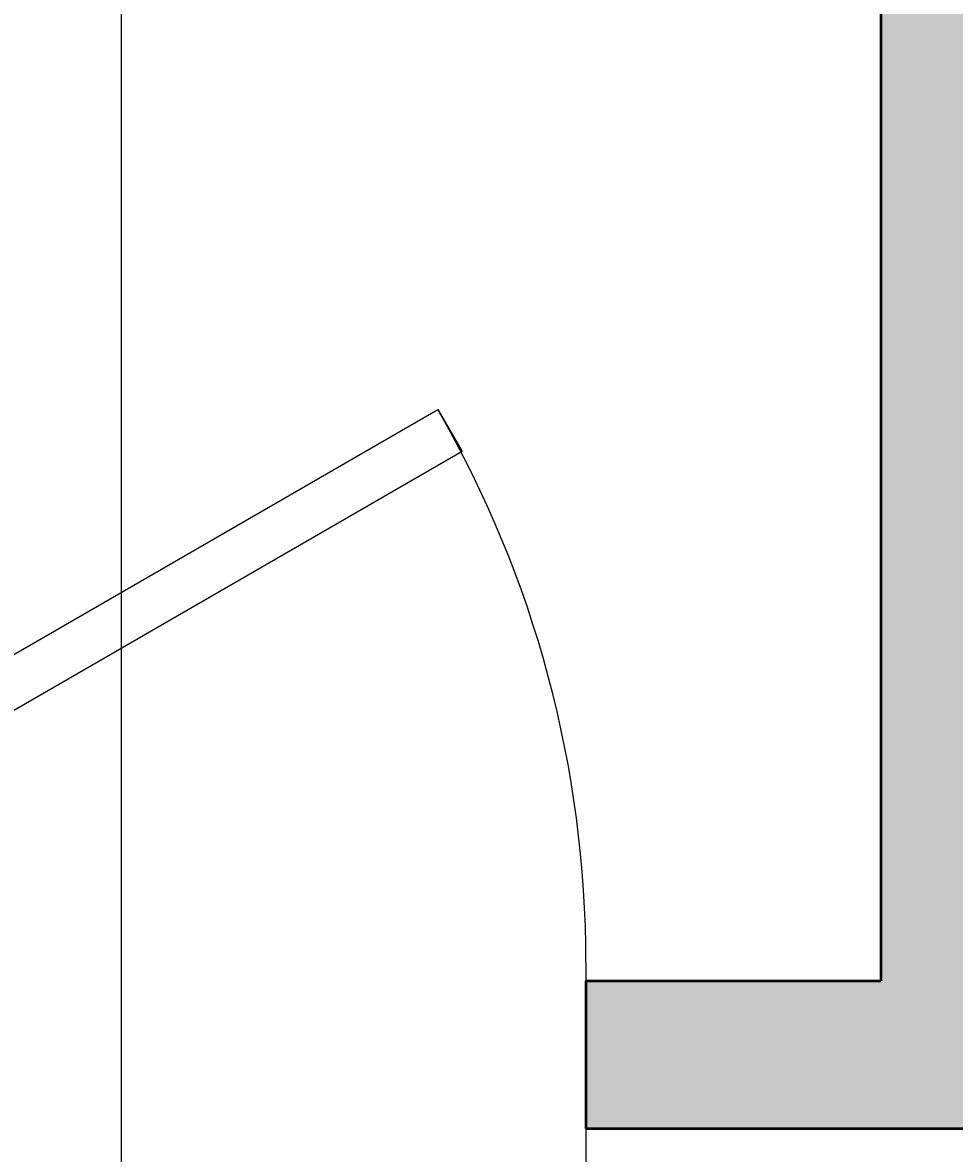
# Model space of a CAD drawing. Units: inches. Extents: x 2231 to 2461, y 2045 to 2455.
# Tile 56 of 95: x 2346 to 2371, y 2302 to 2333. Entities that reach past the tile are written whole.
import ezdxf

# ---------------------------------------------------------------- set-up
doc = ezdxf.new("R2010")
doc.units = ezdxf.units.IN
for name, color, linetype, lineweight in [('A-ANNO-DIMS', 2, 'Continuous', 18), ('A-DOOR', 3, 'Continuous', 25), ('A-WALL', 7, 'Continuous', 50)]:
    doc.layers.add(name, color=color, linetype=linetype, lineweight=lineweight)
doc.layers.add('A-WALL-PATT', color=18, linetype='Continuous', lineweight=13, true_color=0x000000)
doc.styles.get("Standard").update_dxf_attribs({"font": 'arial.ttf'})
doc.dimstyles.get("Standard").update_dxf_attribs({"dimtxt": 0.18, "dimasz": 0.18, "dimexe": 0.18, "dimexo": 0.0625, "dimgap": 0.09, "dimtad": 0, "dimtih": 1, "dimtoh": 1, "dimdec": 4, "dimzin": 0, "dimdsep": 46, "dimtxsty": 'Standard', "dimcen": 0.09, "dimadec": 0, "dimazin": 0, "dimtfac": 1, "dimtdec": 4, "dimtofl": 0, "dimtmove": 0, "dimatfit": 3, "dimfxl": 1, "dimtolj": 1, "dimtzin": 0, "dimarcsym": 0})

# ---------------------------------------------------------------- blocks, each defined once
blk = doc.blocks.new('*U3')
for p, q in [((0, 0), (0, -6)), ((40, 0), (40, -6))]:
    blk.add_line(p, q)
blk.add_lwpolyline([(0, 0), (34.641, 20), (35.516, 18.484), (0.875, -1.516)], close=True)
blk.add_arc((0, 0), 40, 0, 30)
blk = doc.blocks.new('*D52')
at = {"layer": 'A-ANNO-DIMS', "color": 0, "lineweight": -2, "transparency": 16777216}
for p, q in [((2330.794, 2306.77), (2330.794, 2044.803)), ((2360.794, 2306.77), (2360.794, 2044.803)), ((2330.974, 2044.983), (2345.575, 2044.983)), ((2360.614, 2044.983), (2346.012, 2044.983))]:
    blk.add_line(p, q, dxfattribs=at)
at = {"layer": 'A-ANNO-DIMS', "color": 0, "transparency": 16777216}
for points in [[(2330.974, 2045.013), (2330.974, 2044.953), (2330.794, 2044.983)], [(2360.614, 2045.013), (2360.614, 2044.953), (2360.794, 2044.983)]]:
    blk.add_solid(points, dxfattribs=at)
at = {"layer": 'Defpoints', "color": 0, "transparency": 16777216}
for p in [(2330.794, 2306.833), (2360.794, 2306.833), (2360.794, 2044.983)]:
    blk.add_point(p, dxfattribs=at)
at = {"layer": 'A-ANNO-DIMS', "color": 0, "transparency": 16777216, "insert": (2345.794, 2044.983), "char_height": 0.18, "attachment_point": 5}
blk.add_mtext('\\A1;30', dxfattribs=at)
blk = doc.blocks.new('*D66')
at = {"layer": 'A-ANNO-DIMS', "color": 0, "lineweight": -2, "transparency": 16777216}
for p, q in [((2348.189, 2096.895), (2348.189, 2454.645)), ((2348.369, 2454.465), (2378.167, 2454.465)), ((2408.614, 2454.465), (2378.815, 2454.465)), ((2408.794, 2096.895), (2408.794, 2454.645))]:
    blk.add_line(p, q, dxfattribs=at)
at = {"layer": 'A-ANNO-DIMS', "color": 0, "transparency": 16777216}
for points in [[(2348.369, 2454.495), (2348.369, 2454.435), (2348.189, 2454.465)], [(2408.614, 2454.495), (2408.614, 2454.435), (2408.794, 2454.465)]]:
    blk.add_solid(points, dxfattribs=at)
at = {"layer": 'Defpoints', "color": 0, "transparency": 16777216}
for p in [(2408.794, 2454.465), (2348.189, 2096.833), (2408.794, 2096.833)]:
    blk.add_point(p, dxfattribs=at)
at = {"layer": 'A-ANNO-DIMS', "color": 0, "transparency": 16777216, "insert": (2378.491, 2454.465), "char_height": 0.18, "attachment_point": 5}
blk.add_mtext('\\A1;60.6', dxfattribs=at)

msp = doc.modelspace()

# ---------------------------------------------------------------- hatches: boundary and pattern name
at = {"layer": 'A-WALL-PATT'}
h = msp.add_hatch(color=256, dxfattribs=at)
h.dxf.hatch_style = 1
h.paths.add_polyline_path([(2441.7935, 2269.1535), (2432.7935, 2269.1535), (2432.7935, 2186.8328), (2396.7935, 2186.8328), (2396.7935, 2286.8328), (2394.7935, 2286.8328), (2394.7935, 2186.8328), (2334.7935, 2186.8328), (2334.7935, 2182.8328), (2432.7935, 2182.8328), (2432.7935, 2072.8328), (2416.6639, 2072.8328), (2416.6639, 2063.8328), (2441.7935, 2063.8328)])
h.paths.add_polyline_path([(2368.6639, 2072.8328), (2367.04, 2072.8328), (2330.7942, 2072.8328), (2330.7397, 2063.8328), (2368.6639, 2063.8328)])
h.paths.add_polyline_path([(2300.7392, 2068.3328), (2300.7392, 2072.8328), (2298.7935, 2072.8328), (2294.7935, 2072.8328), (2258.7935, 2072.8328), (2258.7935, 2120.8328), (2294.7935, 2120.8328), (2298.7935, 2120.8328), (2298.7935, 2128.8328), (2294.7935, 2128.8328), (2294.7935, 2124.8328), (2258.7935, 2124.8328), (2258.7935, 2182.8328), (2294.7935, 2182.8328), (2294.7935, 2174.8328), (2298.7935, 2174.8328), (2298.7935, 2182.8328), (2304.7935, 2182.8328), (2304.7935, 2186.8328), (2258.7935, 2186.8328), (2258.7935, 2221.999), (2249.7935, 2221.999), (2249.7935, 2063.8328), (2300.7392, 2063.8328)])
h.paths.add_polyline_path([(2391.9338, 2435.8328), (2333.82, 2435.8328), (2333.82, 2426.8328), (2368.7935, 2426.8328), (2368.7935, 2374.9508), (2368.7935, 2370.8328), (2372.3935, 2370.8328), (2372.7935, 2370.8328), (2372.7935, 2426.8328), (2391.9338, 2426.8328)])
h.paths.add_polyline_path([(2441.7935, 2435.8328), (2415.9338, 2435.8328), (2415.9338, 2426.8328), (2432.7935, 2426.8328), (2432.7935, 2334.8328), (2372.7935, 2334.8328), (2372.7935, 2346.8328), (2368.7935, 2346.8328), (2368.7935, 2306.8328), (2360.7935, 2306.8328), (2360.7935, 2302.8328), (2368.7935, 2302.8328), (2372.7935, 2302.8328), (2372.7935, 2330.8328), (2432.7935, 2330.8328), (2432.7935, 2317.1535), (2441.7935, 2317.1535)])
h.paths.add_polyline_path([(2285.82, 2435.8328), (2249.7935, 2435.8328), (2249.7935, 2269.999), (2258.7935, 2269.999), (2258.7935, 2302.8328), (2318.8168, 2302.8328), (2330.7935, 2302.8328), (2330.7935, 2306.8328), (2258.7935, 2306.8328), (2258.7935, 2426.8328), (2285.82, 2426.8328)])

# ---------------------------------------------------------------- linework, layer by layer
at = {"layer": 'A-WALL'}
for p, q in [((2368.7935, 2346.8328), (2368.7935, 2306.8328)), ((2360.7935, 2306.8328), (2360.7935, 2302.8328)), ((2360.7935, 2306.8328), (2368.7935, 2306.8328)), ((2360.7935, 2302.8328), (2368.7935, 2302.8328)), ((2368.7935, 2302.8328), (2372.7935, 2302.8328))]:
    msp.add_line(p, q, dxfattribs=at)

# ---------------------------------------------------------------- block references
at = {"layer": 'A-DOOR', "xscale": 0.75, "yscale": 0.75, "zscale": 0.75}
msp.add_blockref('*U3', (2330.7935, 2307.3328), dxfattribs=at)

# ---------------------------------------------------------------- dimensions: what is measured, and where the dimension line sits
at = {"layer": 'A-ANNO-DIMS'}
for base, p1, p2, override, picture, middle in [((2408.7935, 2454.4653), (2348.1888, 2096.8328), (2408.7935, 2096.8328), {"dimdec": 1, "dimlfac": 1, "dimrnd": 0, "dimzin": 0, "dimdsep": 46, "dimlunit": 2}, '*D66', (2378.4912, 2454.4653)), ((2360.7935, 2044.9825), (2330.7935, 2306.8328), (2360.7935, 2306.8328), {"dimdec": 0, "dimlfac": 1, "dimrnd": 0, "dimzin": 0, "dimdsep": 46, "dimlunit": 2}, '*D52', (2345.7935, 2044.9825))]:
    dim = msp.add_linear_dim(base=base, p1=p1, p2=p2, dimstyle='Standard', override=override, dxfattribs=at)
    dim.commit()
    dim.dimension.update_dxf_attribs({"geometry": picture, "text_midpoint": middle})

doc.saveas('drawing.dxf')
